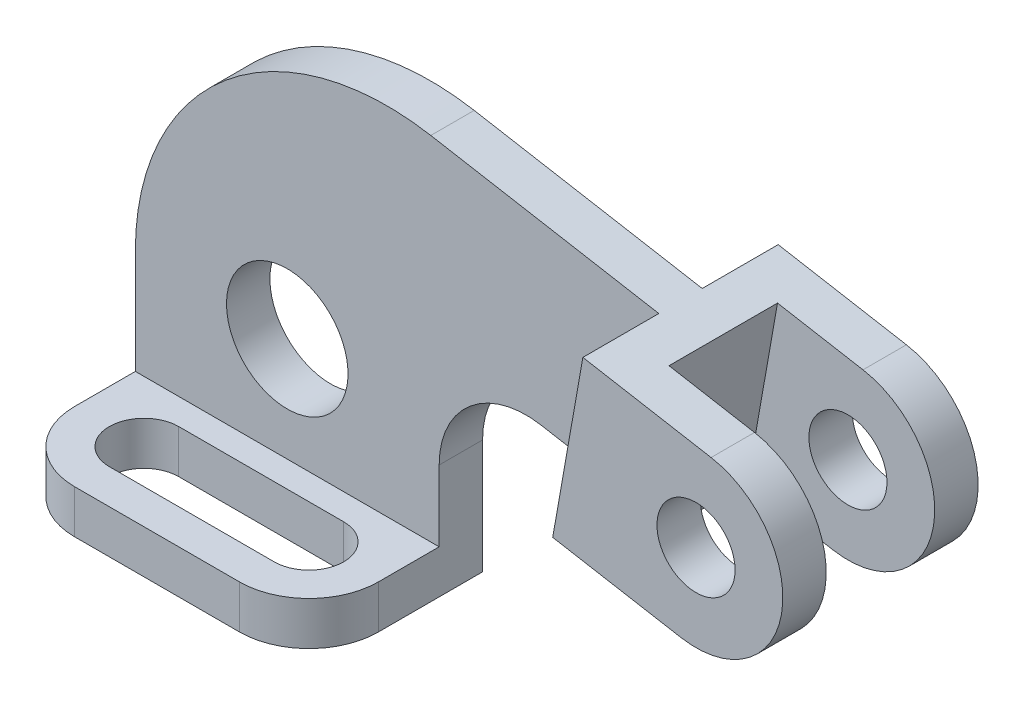
ISO-10303-21;
HEADER;
FILE_DESCRIPTION(('STEP AP214'),'2;1');
FILE_NAME('part.step','',(''),(''),'','','');
FILE_SCHEMA(('AUTOMOTIVE_DESIGN { 1 0 10303 214 1 1 1 1 }'));
ENDSEC;
DATA;
#1=APPLICATION_CONTEXT('core data for automotive mechanical design processes');
#2=APPLICATION_PROTOCOL_DEFINITION('international standard','automotive_design',2000,#1);
#3=PRODUCT_CONTEXT('',#1,'mechanical');
#4=PRODUCT('Part','Part','',(#3));
#5=PRODUCT_RELATED_PRODUCT_CATEGORY('part','',(#4));
#6=PRODUCT_DEFINITION_FORMATION('','',#4);
#7=PRODUCT_DEFINITION_CONTEXT('part definition',#1,'design');
#8=PRODUCT_DEFINITION('design','',#6,#7);
#9=PRODUCT_DEFINITION_SHAPE('','',#8);
#10=(LENGTH_UNIT() NAMED_UNIT(*) SI_UNIT(.MILLI.,.METRE.));
#11=(NAMED_UNIT(*) PLANE_ANGLE_UNIT() SI_UNIT($,.RADIAN.));
#12=(NAMED_UNIT(*) SI_UNIT($,.STERADIAN.) SOLID_ANGLE_UNIT());
#13=UNCERTAINTY_MEASURE_WITH_UNIT(LENGTH_MEASURE(1.E-05),#10,'distance_accuracy_value','');
#14=(GEOMETRIC_REPRESENTATION_CONTEXT(3) GLOBAL_UNCERTAINTY_ASSIGNED_CONTEXT((#13)) GLOBAL_UNIT_ASSIGNED_CONTEXT((#10,
#11,#12)) REPRESENTATION_CONTEXT('',''));
#15=CARTESIAN_POINT('',(0.,0.,0.));
#16=DIRECTION('',(0.,0.,1.));
#17=DIRECTION('',(1.,0.,0.));
#18=AXIS2_PLACEMENT_3D('',#15,#16,#17);
#19=CARTESIAN_POINT('',(-54.,10.,14.));
#20=DIRECTION('',(0.,1.,0.));
#21=DIRECTION('',(0.,0.,1.));
#22=AXIS2_PLACEMENT_3D('',#19,#20,#21);
#23=PLANE('',#22);
#24=DIRECTION('',(0.,0.,-1.));
#25=VECTOR('',#24,1.);
#26=CARTESIAN_POINT('',(0.,10.,13.9999999999999));
#27=LINE('',#26,#25);
#28=CARTESIAN_POINT('',(0.,10.,13.9999999999999));
#29=VERTEX_POINT('',#28);
#30=CARTESIAN_POINT('',(0.,10.,0.));
#31=VERTEX_POINT('',#30);
#32=EDGE_CURVE('E341',#29,#31,#27,.T.);
#33=ORIENTED_EDGE('',*,*,#32,.T.);
#34=DIRECTION('',(-1.,0.,0.));
#35=VECTOR('',#34,1.);
#36=CARTESIAN_POINT('',(0.,10.,0.));
#37=LINE('',#36,#35);
#38=CARTESIAN_POINT('',(-70.,10.,0.));
#39=VERTEX_POINT('',#38);
#40=EDGE_CURVE('E350',#31,#39,#37,.T.);
#41=ORIENTED_EDGE('',*,*,#40,.T.);
#42=DIRECTION('',(0.,0.,1.));
#43=VECTOR('',#42,1.);
#44=CARTESIAN_POINT('',(-70.,10.,0.));
#45=LINE('',#44,#43);
#46=CARTESIAN_POINT('',(-70.,10.,14.));
#47=VERTEX_POINT('',#46);
#48=EDGE_CURVE('E351',#39,#47,#45,.T.);
#49=ORIENTED_EDGE('',*,*,#48,.T.);
#50=CARTESIAN_POINT('',(-54.,10.,14.));
#51=DIRECTION('',(0.,1.,0.));
#52=DIRECTION('',(0.,0.,1.));
#53=AXIS2_PLACEMENT_3D('',#50,#51,#52);
#54=CIRCLE('',#53,16.);
#55=CARTESIAN_POINT('',(-54.,10.,30.));
#56=VERTEX_POINT('',#55);
#57=EDGE_CURVE('E354',#47,#56,#54,.T.);
#58=ORIENTED_EDGE('',*,*,#57,.T.);
#59=DIRECTION('',(1.,0.,0.));
#60=VECTOR('',#59,1.);
#61=CARTESIAN_POINT('',(-54.,10.,30.));
#62=LINE('',#61,#60);
#63=CARTESIAN_POINT('',(-16.0000000000001,10.,30.));
#64=VERTEX_POINT('',#63);
#65=EDGE_CURVE('E355',#56,#64,#62,.T.);
#66=ORIENTED_EDGE('',*,*,#65,.T.);
#67=CARTESIAN_POINT('',(-16.,10.,14.));
#68=DIRECTION('',(0.,1.,0.));
#69=DIRECTION('',(0.,0.,1.));
#70=AXIS2_PLACEMENT_3D('',#67,#68,#69);
#71=CIRCLE('',#70,16.);
#72=EDGE_CURVE('E360',#64,#29,#71,.T.);
#73=ORIENTED_EDGE('',*,*,#72,.T.);
#74=EDGE_LOOP('',(#33,#41,#49,#58,#66,#73));
#75=FACE_BOUND('',#74,.T.);
#76=DIRECTION('',(1.,0.,0.));
#77=VECTOR('',#76,1.);
#78=CARTESIAN_POINT('',(-54.,10.,22.));
#79=LINE('',#78,#77);
#80=CARTESIAN_POINT('',(-54.,10.,22.));
#81=VERTEX_POINT('',#80);
#82=CARTESIAN_POINT('',(-16.,10.,22.));
#83=VERTEX_POINT('',#82);
#84=EDGE_CURVE('E319',#81,#83,#79,.T.);
#85=ORIENTED_EDGE('',*,*,#84,.F.);
#86=CARTESIAN_POINT('',(-54.,10.,14.));
#87=DIRECTION('',(0.,1.,0.));
#88=DIRECTION('',(0.,0.,1.));
#89=AXIS2_PLACEMENT_3D('',#86,#87,#88);
#90=CIRCLE('',#89,8.);
#91=CARTESIAN_POINT('',(-54.,10.,6.00000000000001));
#92=VERTEX_POINT('',#91);
#93=EDGE_CURVE('E318',#92,#81,#90,.T.);
#94=ORIENTED_EDGE('',*,*,#93,.F.);
#95=DIRECTION('',(-1.,0.,0.));
#96=VECTOR('',#95,1.);
#97=CARTESIAN_POINT('',(-54.,10.,6.00000000000001));
#98=LINE('',#97,#96);
#99=CARTESIAN_POINT('',(-16.,10.,6.00000000000001));
#100=VERTEX_POINT('',#99);
#101=EDGE_CURVE('E324',#100,#92,#98,.T.);
#102=ORIENTED_EDGE('',*,*,#101,.F.);
#103=CARTESIAN_POINT('',(-16.,10.,14.));
#104=DIRECTION('',(0.,1.,0.));
#105=DIRECTION('',(0.,0.,1.));
#106=AXIS2_PLACEMENT_3D('',#103,#104,#105);
#107=CIRCLE('',#106,8.);
#108=EDGE_CURVE('E323',#83,#100,#107,.T.);
#109=ORIENTED_EDGE('',*,*,#108,.F.);
#110=EDGE_LOOP('',(#85,#94,#102,#109));
#111=FACE_BOUND('',#110,.T.);
#112=ADVANCED_FACE('F39',(#75,#111),#23,.T.);
#113=CARTESIAN_POINT('',(-54.,0.,14.));
#114=DIRECTION('',(0.,1.,0.));
#115=DIRECTION('',(0.,0.,1.));
#116=AXIS2_PLACEMENT_3D('',#113,#114,#115);
#117=PLANE('',#116);
#118=DIRECTION('',(0.,0.,-1.));
#119=VECTOR('',#118,1.);
#120=CARTESIAN_POINT('',(0.,0.,13.9999999999999));
#121=LINE('',#120,#119);
#122=CARTESIAN_POINT('',(0.,0.,13.9999999999999));
#123=VERTEX_POINT('',#122);
#124=CARTESIAN_POINT('',(0.,0.,-10.));
#125=VERTEX_POINT('',#124);
#126=EDGE_CURVE('E344',#123,#125,#121,.T.);
#127=ORIENTED_EDGE('',*,*,#126,.F.);
#128=CARTESIAN_POINT('',(-16.,0.,14.));
#129=DIRECTION('',(0.,1.,0.));
#130=DIRECTION('',(0.,0.,1.));
#131=AXIS2_PLACEMENT_3D('',#128,#129,#130);
#132=CIRCLE('',#131,16.);
#133=CARTESIAN_POINT('',(-16.0000000000001,0.,30.));
#134=VERTEX_POINT('',#133);
#135=EDGE_CURVE('E346',#134,#123,#132,.T.);
#136=ORIENTED_EDGE('',*,*,#135,.F.);
#137=DIRECTION('',(1.,0.,0.));
#138=VECTOR('',#137,1.);
#139=CARTESIAN_POINT('',(-54.,0.,30.));
#140=LINE('',#139,#138);
#141=CARTESIAN_POINT('',(-54.,0.,30.));
#142=VERTEX_POINT('',#141);
#143=EDGE_CURVE('E364',#142,#134,#140,.T.);
#144=ORIENTED_EDGE('',*,*,#143,.F.);
#145=CARTESIAN_POINT('',(-54.,0.,14.));
#146=DIRECTION('',(0.,1.,0.));
#147=DIRECTION('',(0.,0.,1.));
#148=AXIS2_PLACEMENT_3D('',#145,#146,#147);
#149=CIRCLE('',#148,16.);
#150=CARTESIAN_POINT('',(-70.,0.,14.));
#151=VERTEX_POINT('',#150);
#152=EDGE_CURVE('E361',#151,#142,#149,.T.);
#153=ORIENTED_EDGE('',*,*,#152,.F.);
#154=DIRECTION('',(0.,0.,1.));
#155=VECTOR('',#154,1.);
#156=CARTESIAN_POINT('',(-70.,0.,0.));
#157=LINE('',#156,#155);
#158=CARTESIAN_POINT('',(-70.,0.,-9.99999999999999));
#159=VERTEX_POINT('',#158);
#160=EDGE_CURVE('E363',#159,#151,#157,.T.);
#161=ORIENTED_EDGE('',*,*,#160,.F.);
#162=DIRECTION('',(-1.,0.,0.));
#163=VECTOR('',#162,1.);
#164=CARTESIAN_POINT('',(-70.,0.,-9.99999999999999));
#165=LINE('',#164,#163);
#166=EDGE_CURVE('E271',#125,#159,#165,.T.);
#167=ORIENTED_EDGE('',*,*,#166,.F.);
#168=EDGE_LOOP('',(#127,#136,#144,#153,#161,#167));
#169=FACE_BOUND('',#168,.T.);
#170=CARTESIAN_POINT('',(-54.,0.,14.));
#171=DIRECTION('',(0.,1.,0.));
#172=DIRECTION('',(0.,0.,1.));
#173=AXIS2_PLACEMENT_3D('',#170,#171,#172);
#174=CIRCLE('',#173,8.);
#175=CARTESIAN_POINT('',(-54.,0.,6.00000000000001));
#176=VERTEX_POINT('',#175);
#177=CARTESIAN_POINT('',(-54.,0.,22.));
#178=VERTEX_POINT('',#177);
#179=EDGE_CURVE('E62',#176,#178,#174,.T.);
#180=ORIENTED_EDGE('',*,*,#179,.T.);
#181=DIRECTION('',(1.,0.,0.));
#182=VECTOR('',#181,1.);
#183=CARTESIAN_POINT('',(-54.,0.,22.));
#184=LINE('',#183,#182);
#185=CARTESIAN_POINT('',(-16.,0.,22.));
#186=VERTEX_POINT('',#185);
#187=EDGE_CURVE('E328',#178,#186,#184,.T.);
#188=ORIENTED_EDGE('',*,*,#187,.T.);
#189=CARTESIAN_POINT('',(-16.,0.,14.));
#190=DIRECTION('',(0.,1.,0.));
#191=DIRECTION('',(0.,0.,1.));
#192=AXIS2_PLACEMENT_3D('',#189,#190,#191);
#193=CIRCLE('',#192,8.);
#194=CARTESIAN_POINT('',(-16.,0.,6.00000000000001));
#195=VERTEX_POINT('',#194);
#196=EDGE_CURVE('E335',#186,#195,#193,.T.);
#197=ORIENTED_EDGE('',*,*,#196,.T.);
#198=DIRECTION('',(-1.,0.,0.));
#199=VECTOR('',#198,1.);
#200=CARTESIAN_POINT('',(-54.,0.,6.00000000000001));
#201=LINE('',#200,#199);
#202=EDGE_CURVE('E321',#195,#176,#201,.T.);
#203=ORIENTED_EDGE('',*,*,#202,.T.);
#204=EDGE_LOOP('',(#180,#188,#197,#203));
#205=FACE_BOUND('',#204,.T.);
#206=ADVANCED_FACE('F384',(#169,#205),#117,.F.);
#207=CARTESIAN_POINT('',(0.,10.,13.9999999999999));
#208=DIRECTION('',(-1.,0.,0.));
#209=DIRECTION('',(0.,0.,1.));
#210=AXIS2_PLACEMENT_3D('',#207,#208,#209);
#211=PLANE('',#210);
#212=ORIENTED_EDGE('',*,*,#126,.T.);
#213=DIRECTION('',(0.,-1.,0.));
#214=VECTOR('',#213,1.);
#215=CARTESIAN_POINT('',(0.,0.,-10.));
#216=LINE('',#215,#214);
#217=CARTESIAN_POINT('',(0.,26.3266833935575,-10.));
#218=VERTEX_POINT('',#217);
#219=EDGE_CURVE('E286',#218,#125,#216,.T.);
#220=ORIENTED_EDGE('',*,*,#219,.F.);
#221=DIRECTION('',(0.,0.,1.));
#222=VECTOR('',#221,1.);
#223=CARTESIAN_POINT('',(0.,26.3266833935575,-10.));
#224=LINE('',#223,#222);
#225=CARTESIAN_POINT('',(0.,26.3266833935575,0.));
#226=VERTEX_POINT('',#225);
#227=EDGE_CURVE('E295',#218,#226,#224,.T.);
#228=ORIENTED_EDGE('',*,*,#227,.T.);
#229=DIRECTION('',(0.,-1.,0.));
#230=VECTOR('',#229,1.);
#231=CARTESIAN_POINT('',(0.,0.,0.));
#232=LINE('',#231,#230);
#233=EDGE_CURVE('E274',#226,#31,#232,.T.);
#234=ORIENTED_EDGE('',*,*,#233,.T.);
#235=ORIENTED_EDGE('',*,*,#32,.F.);
#236=DIRECTION('',(0.,-1.,0.));
#237=VECTOR('',#236,1.);
#238=CARTESIAN_POINT('',(0.,10.,13.9999999999999));
#239=LINE('',#238,#237);
#240=EDGE_CURVE('E356',#29,#123,#239,.T.);
#241=ORIENTED_EDGE('',*,*,#240,.T.);
#242=EDGE_LOOP('',(#212,#220,#228,#234,#235,#241));
#243=FACE_BOUND('',#242,.T.);
#244=ADVANCED_FACE('F41',(#243),#211,.F.);
#245=CARTESIAN_POINT('',(-70.,10.,0.));
#246=DIRECTION('',(1.,0.,0.));
#247=DIRECTION('',(0.,0.,-1.));
#248=AXIS2_PLACEMENT_3D('',#245,#246,#247);
#249=PLANE('',#248);
#250=ORIENTED_EDGE('',*,*,#160,.T.);
#251=DIRECTION('',(0.,-1.,0.));
#252=VECTOR('',#251,1.);
#253=CARTESIAN_POINT('',(-70.,10.,14.));
#254=LINE('',#253,#252);
#255=EDGE_CURVE('E11',#47,#151,#254,.T.);
#256=ORIENTED_EDGE('',*,*,#255,.F.);
#257=ORIENTED_EDGE('',*,*,#48,.F.);
#258=DIRECTION('',(0.,1.,0.));
#259=VECTOR('',#258,1.);
#260=CARTESIAN_POINT('',(-70.,0.,0.));
#261=LINE('',#260,#259);
#262=CARTESIAN_POINT('',(-70.,34.,0.));
#263=VERTEX_POINT('',#262);
#264=EDGE_CURVE('E268',#39,#263,#261,.T.);
#265=ORIENTED_EDGE('',*,*,#264,.T.);
#266=DIRECTION('',(0.,0.,1.));
#267=VECTOR('',#266,1.);
#268=CARTESIAN_POINT('',(-70.,34.,-9.99999999999999));
#269=LINE('',#268,#267);
#270=CARTESIAN_POINT('',(-70.,34.,-9.99999999999999));
#271=VERTEX_POINT('',#270);
#272=EDGE_CURVE('E312',#271,#263,#269,.T.);
#273=ORIENTED_EDGE('',*,*,#272,.F.);
#274=DIRECTION('',(0.,1.,0.));
#275=VECTOR('',#274,1.);
#276=CARTESIAN_POINT('',(-70.,0.,-9.99999999999999));
#277=LINE('',#276,#275);
#278=EDGE_CURVE('E273',#159,#271,#277,.T.);
#279=ORIENTED_EDGE('',*,*,#278,.F.);
#280=EDGE_LOOP('',(#250,#256,#257,#265,#273,#279));
#281=FACE_BOUND('',#280,.T.);
#282=ADVANCED_FACE('F405',(#281),#249,.F.);
#283=CARTESIAN_POINT('',(-54.,10.,14.));
#284=DIRECTION('',(0.,-1.,0.));
#285=DIRECTION('',(0.,0.,-1.));
#286=AXIS2_PLACEMENT_3D('',#283,#284,#285);
#287=CYLINDRICAL_SURFACE('',#286,16.);
#288=ORIENTED_EDGE('',*,*,#152,.T.);
#289=DIRECTION('',(0.,-1.,0.));
#290=VECTOR('',#289,1.);
#291=CARTESIAN_POINT('',(-54.,10.,30.));
#292=LINE('',#291,#290);
#293=EDGE_CURVE('E50',#56,#142,#292,.T.);
#294=ORIENTED_EDGE('',*,*,#293,.F.);
#295=ORIENTED_EDGE('',*,*,#57,.F.);
#296=ORIENTED_EDGE('',*,*,#255,.T.);
#297=EDGE_LOOP('',(#288,#294,#295,#296));
#298=FACE_BOUND('',#297,.T.);
#299=ADVANCED_FACE('F398',(#298),#287,.T.);
#300=CARTESIAN_POINT('',(-54.,10.,30.));
#301=DIRECTION('',(0.,0.,-1.));
#302=DIRECTION('',(-1.,0.,0.));
#303=AXIS2_PLACEMENT_3D('',#300,#301,#302);
#304=PLANE('',#303);
#305=ORIENTED_EDGE('',*,*,#143,.T.);
#306=DIRECTION('',(0.,-1.,0.));
#307=VECTOR('',#306,1.);
#308=CARTESIAN_POINT('',(-16.0000000000001,10.,30.));
#309=LINE('',#308,#307);
#310=EDGE_CURVE('E367',#64,#134,#309,.T.);
#311=ORIENTED_EDGE('',*,*,#310,.F.);
#312=ORIENTED_EDGE('',*,*,#65,.F.);
#313=ORIENTED_EDGE('',*,*,#293,.T.);
#314=EDGE_LOOP('',(#305,#311,#312,#313));
#315=FACE_BOUND('',#314,.T.);
#316=ADVANCED_FACE('F380',(#315),#304,.F.);
#317=CARTESIAN_POINT('',(-16.,10.,14.));
#318=DIRECTION('',(0.,-1.,0.));
#319=DIRECTION('',(0.,0.,-1.));
#320=AXIS2_PLACEMENT_3D('',#317,#318,#319);
#321=CYLINDRICAL_SURFACE('',#320,16.);
#322=ORIENTED_EDGE('',*,*,#135,.T.);
#323=ORIENTED_EDGE('',*,*,#240,.F.);
#324=ORIENTED_EDGE('',*,*,#72,.F.);
#325=ORIENTED_EDGE('',*,*,#310,.T.);
#326=EDGE_LOOP('',(#322,#323,#324,#325));
#327=FACE_BOUND('',#326,.T.);
#328=ADVANCED_FACE('F388',(#327),#321,.T.);
#329=CARTESIAN_POINT('',(-54.,10.,14.));
#330=DIRECTION('',(0.,-1.,0.));
#331=DIRECTION('',(0.,0.,-1.));
#332=AXIS2_PLACEMENT_3D('',#329,#330,#331);
#333=CYLINDRICAL_SURFACE('',#332,8.);
#334=ORIENTED_EDGE('',*,*,#179,.F.);
#335=DIRECTION('',(0.,-1.,0.));
#336=VECTOR('',#335,1.);
#337=CARTESIAN_POINT('',(-54.,10.,6.00000000000001));
#338=LINE('',#337,#336);
#339=EDGE_CURVE('E330',#92,#176,#338,.T.);
#340=ORIENTED_EDGE('',*,*,#339,.F.);
#341=ORIENTED_EDGE('',*,*,#93,.T.);
#342=DIRECTION('',(0.,-1.,0.));
#343=VECTOR('',#342,1.);
#344=CARTESIAN_POINT('',(-54.,10.,22.));
#345=LINE('',#344,#343);
#346=EDGE_CURVE('E342',#81,#178,#345,.T.);
#347=ORIENTED_EDGE('',*,*,#346,.T.);
#348=EDGE_LOOP('',(#334,#340,#341,#347));
#349=FACE_BOUND('',#348,.T.);
#350=ADVANCED_FACE('F495',(#349),#333,.F.);
#351=CARTESIAN_POINT('',(-54.,10.,22.));
#352=DIRECTION('',(0.,0.,-1.));
#353=DIRECTION('',(-1.,0.,0.));
#354=AXIS2_PLACEMENT_3D('',#351,#352,#353);
#355=PLANE('',#354);
#356=ORIENTED_EDGE('',*,*,#187,.F.);
#357=ORIENTED_EDGE('',*,*,#346,.F.);
#358=ORIENTED_EDGE('',*,*,#84,.T.);
#359=DIRECTION('',(0.,-1.,0.));
#360=VECTOR('',#359,1.);
#361=CARTESIAN_POINT('',(-16.,10.,22.));
#362=LINE('',#361,#360);
#363=EDGE_CURVE('E338',#83,#186,#362,.T.);
#364=ORIENTED_EDGE('',*,*,#363,.T.);
#365=EDGE_LOOP('',(#356,#357,#358,#364));
#366=FACE_BOUND('',#365,.T.);
#367=ADVANCED_FACE('F534',(#366),#355,.T.);
#368=CARTESIAN_POINT('',(-16.,10.,14.));
#369=DIRECTION('',(0.,-1.,0.));
#370=DIRECTION('',(0.,0.,-1.));
#371=AXIS2_PLACEMENT_3D('',#368,#369,#370);
#372=CYLINDRICAL_SURFACE('',#371,8.);
#373=ORIENTED_EDGE('',*,*,#196,.F.);
#374=ORIENTED_EDGE('',*,*,#363,.F.);
#375=ORIENTED_EDGE('',*,*,#108,.T.);
#376=DIRECTION('',(0.,-1.,0.));
#377=VECTOR('',#376,1.);
#378=CARTESIAN_POINT('',(-16.,10.,6.00000000000001));
#379=LINE('',#378,#377);
#380=EDGE_CURVE('E53',#100,#195,#379,.T.);
#381=ORIENTED_EDGE('',*,*,#380,.T.);
#382=EDGE_LOOP('',(#373,#374,#375,#381));
#383=FACE_BOUND('',#382,.T.);
#384=ADVANCED_FACE('F521',(#383),#372,.F.);
#385=CARTESIAN_POINT('',(-54.,10.,6.00000000000001));
#386=DIRECTION('',(0.,0.,1.));
#387=DIRECTION('',(1.,0.,0.));
#388=AXIS2_PLACEMENT_3D('',#385,#386,#387);
#389=PLANE('',#388);
#390=ORIENTED_EDGE('',*,*,#202,.F.);
#391=ORIENTED_EDGE('',*,*,#380,.F.);
#392=ORIENTED_EDGE('',*,*,#101,.T.);
#393=ORIENTED_EDGE('',*,*,#339,.T.);
#394=EDGE_LOOP('',(#390,#391,#392,#393));
#395=FACE_BOUND('',#394,.T.);
#396=ADVANCED_FACE('F518',(#395),#389,.T.);
#397=CARTESIAN_POINT('',(20.,26.3266833935575,-10.));
#398=DIRECTION('',(0.,0.,-1.));
#399=DIRECTION('',(-1.,0.,0.));
#400=AXIS2_PLACEMENT_3D('',#397,#398,#399);
#401=PLANE('',#400);
#402=ORIENTED_EDGE('',*,*,#166,.T.);
#403=ORIENTED_EDGE('',*,*,#278,.T.);
#404=CARTESIAN_POINT('',(-12.,34.,-10.));
#405=DIRECTION('',(0.,0.,-1.));
#406=DIRECTION('',(-1.,0.,0.));
#407=AXIS2_PLACEMENT_3D('',#404,#405,#406);
#408=CIRCLE('',#407,58.);
#409=CARTESIAN_POINT('',(-1.92840569531779,91.118849674708,-10.));
#410=VERTEX_POINT('',#409);
#411=EDGE_CURVE('E280',#271,#410,#408,.T.);
#412=ORIENTED_EDGE('',*,*,#411,.T.);
#413=DIRECTION('',(0.984807753012207,-0.173648177666935,0.));
#414=VECTOR('',#413,1.);
#415=CARTESIAN_POINT('',(-1.92840569531779,91.118849674708,-10.));
#416=LINE('',#415,#414);
#417=CARTESIAN_POINT('',(50.610518394572,81.8548198202663,-10.));
#418=VERTEX_POINT('',#417);
#419=EDGE_CURVE('E276',#410,#418,#416,.T.);
#420=ORIENTED_EDGE('',*,*,#419,.T.);
#421=DIRECTION('',(-0.173648177666935,-0.984807753012207,0.));
#422=VECTOR('',#421,1.);
#423=CARTESIAN_POINT('',(50.610518394572,81.8548198202663,-10.));
#424=LINE('',#423,#422);
#425=CARTESIAN_POINT('',(43.6645912878946,42.462509699778,-10.));
#426=VERTEX_POINT('',#425);
#427=EDGE_CURVE('E282',#418,#426,#424,.T.);
#428=ORIENTED_EDGE('',*,*,#427,.T.);
#429=DIRECTION('',(-0.984807753012207,0.173648177666934,0.));
#430=VECTOR('',#429,1.);
#431=CARTESIAN_POINT('',(23.4729635533387,46.0228384538016,-10.));
#432=LINE('',#431,#430);
#433=CARTESIAN_POINT('',(23.4729635533387,46.0228384538016,-10.));
#434=VERTEX_POINT('',#433);
#435=EDGE_CURVE('E285',#426,#434,#432,.T.);
#436=ORIENTED_EDGE('',*,*,#435,.T.);
#437=CARTESIAN_POINT('',(20.,26.3266833935575,-10.));
#438=DIRECTION('',(0.,0.,1.));
#439=DIRECTION('',(-1.,0.,0.));
#440=AXIS2_PLACEMENT_3D('',#437,#438,#439);
#441=CIRCLE('',#440,20.);
#442=EDGE_CURVE('E290',#434,#218,#441,.T.);
#443=ORIENTED_EDGE('',*,*,#442,.T.);
#444=ORIENTED_EDGE('',*,*,#219,.T.);
#445=EDGE_LOOP('',(#402,#403,#412,#420,#428,#436,#443,#444));
#446=FACE_BOUND('',#445,.T.);
#447=CARTESIAN_POINT('',(-35.,34.,-10.));
#448=DIRECTION('',(0.,0.,-1.));
#449=DIRECTION('',(-1.,0.,0.));
#450=AXIS2_PLACEMENT_3D('',#447,#448,#449);
#451=CIRCLE('',#450,14.);
#452=CARTESIAN_POINT('',(-49.,34.,-9.99999999999999));
#453=VERTEX_POINT('',#452);
#454=EDGE_CURVE('E264',#453,#453,#451,.T.);
#455=ORIENTED_EDGE('',*,*,#454,.F.);
#456=EDGE_LOOP('',(#455));
#457=FACE_BOUND('',#456,.T.);
#458=ADVANCED_FACE('F406',(#446,#457),#401,.T.);
#459=CARTESIAN_POINT('',(20.,26.3266833935575,0.));
#460=DIRECTION('',(0.,0.,-1.));
#461=DIRECTION('',(-1.,0.,0.));
#462=AXIS2_PLACEMENT_3D('',#459,#460,#461);
#463=PLANE('',#462);
#464=ORIENTED_EDGE('',*,*,#40,.F.);
#465=ORIENTED_EDGE('',*,*,#233,.F.);
#466=CARTESIAN_POINT('',(20.,26.3266833935575,0.));
#467=DIRECTION('',(0.,0.,1.));
#468=DIRECTION('',(-1.,0.,0.));
#469=AXIS2_PLACEMENT_3D('',#466,#467,#468);
#470=CIRCLE('',#469,20.);
#471=CARTESIAN_POINT('',(23.4729635533387,46.0228384538016,0.));
#472=VERTEX_POINT('',#471);
#473=EDGE_CURVE('E304',#472,#226,#470,.T.);
#474=ORIENTED_EDGE('',*,*,#473,.F.);
#475=DIRECTION('',(-0.984807753012207,0.173648177666934,0.));
#476=VECTOR('',#475,1.);
#477=CARTESIAN_POINT('',(23.4729635533387,46.0228384538016,0.));
#478=LINE('',#477,#476);
#479=CARTESIAN_POINT('',(43.6645912878946,42.462509699778,0.));
#480=VERTEX_POINT('',#479);
#481=EDGE_CURVE('E302',#480,#472,#478,.T.);
#482=ORIENTED_EDGE('',*,*,#481,.F.);
#483=DIRECTION('',(-0.173648177666935,-0.984807753012207,0.));
#484=VECTOR('',#483,1.);
#485=CARTESIAN_POINT('',(50.610518394572,81.8548198202663,0.));
#486=LINE('',#485,#484);
#487=CARTESIAN_POINT('',(50.610518394572,81.8548198202663,0.));
#488=VERTEX_POINT('',#487);
#489=EDGE_CURVE('E298',#488,#480,#486,.T.);
#490=ORIENTED_EDGE('',*,*,#489,.F.);
#491=DIRECTION('',(0.984807753012207,-0.173648177666935,0.));
#492=VECTOR('',#491,1.);
#493=CARTESIAN_POINT('',(-1.92840569531779,91.118849674708,0.));
#494=LINE('',#493,#492);
#495=CARTESIAN_POINT('',(-1.92840569531779,91.118849674708,0.));
#496=VERTEX_POINT('',#495);
#497=EDGE_CURVE('E296',#496,#488,#494,.T.);
#498=ORIENTED_EDGE('',*,*,#497,.F.);
#499=CARTESIAN_POINT('',(-12.,34.,0.));
#500=DIRECTION('',(0.,0.,-1.));
#501=DIRECTION('',(-1.,0.,0.));
#502=AXIS2_PLACEMENT_3D('',#499,#500,#501);
#503=CIRCLE('',#502,58.);
#504=EDGE_CURVE('E294',#263,#496,#503,.T.);
#505=ORIENTED_EDGE('',*,*,#504,.F.);
#506=ORIENTED_EDGE('',*,*,#264,.F.);
#507=EDGE_LOOP('',(#464,#465,#474,#482,#490,#498,#505,#506));
#508=FACE_BOUND('',#507,.T.);
#509=CARTESIAN_POINT('',(-35.,34.,0.));
#510=DIRECTION('',(0.,0.,-1.));
#511=DIRECTION('',(-1.,0.,0.));
#512=AXIS2_PLACEMENT_3D('',#509,#510,#511);
#513=CIRCLE('',#512,14.);
#514=CARTESIAN_POINT('',(-49.,34.,0.));
#515=VERTEX_POINT('',#514);
#516=EDGE_CURVE('E259',#515,#515,#513,.T.);
#517=ORIENTED_EDGE('',*,*,#516,.T.);
#518=EDGE_LOOP('',(#517));
#519=FACE_BOUND('',#518,.T.);
#520=ADVANCED_FACE('F414',(#508,#519),#463,.F.);
#521=CARTESIAN_POINT('',(-12.,34.,-10.));
#522=DIRECTION('',(0.,0.,1.));
#523=DIRECTION('',(1.,0.,0.));
#524=AXIS2_PLACEMENT_3D('',#521,#522,#523);
#525=CYLINDRICAL_SURFACE('',#524,58.);
#526=ORIENTED_EDGE('',*,*,#504,.T.);
#527=DIRECTION('',(0.,0.,1.));
#528=VECTOR('',#527,1.);
#529=CARTESIAN_POINT('',(-1.92840569531779,91.118849674708,-10.));
#530=LINE('',#529,#528);
#531=EDGE_CURVE('E315',#410,#496,#530,.T.);
#532=ORIENTED_EDGE('',*,*,#531,.F.);
#533=ORIENTED_EDGE('',*,*,#411,.F.);
#534=ORIENTED_EDGE('',*,*,#272,.T.);
#535=EDGE_LOOP('',(#526,#532,#533,#534));
#536=FACE_BOUND('',#535,.T.);
#537=ADVANCED_FACE('F419',(#536),#525,.T.);
#538=CARTESIAN_POINT('',(-1.92840569531779,91.118849674708,-10.));
#539=DIRECTION('',(-0.173648177666935,-0.984807753012207,0.));
#540=DIRECTION('',(0.984807753012207,-0.173648177666935,0.));
#541=AXIS2_PLACEMENT_3D('',#538,#539,#540);
#542=PLANE('',#541);
#543=ORIENTED_EDGE('',*,*,#497,.T.);
#544=DIRECTION('',(0.,0.,1.));
#545=VECTOR('',#544,1.);
#546=CARTESIAN_POINT('',(50.610518394572,81.8548198202663,-27.5));
#547=LINE('',#546,#545);
#548=CARTESIAN_POINT('',(50.6105183945721,81.8548198202663,17.5));
#549=VERTEX_POINT('',#548);
#550=EDGE_CURVE('E239',#488,#549,#547,.T.);
#551=ORIENTED_EDGE('',*,*,#550,.T.);
#552=DIRECTION('',(0.984807753012207,-0.173648177666935,0.));
#553=VECTOR('',#552,1.);
#554=CARTESIAN_POINT('',(50.6105183945721,81.8548198202663,17.5));
#555=LINE('',#554,#553);
#556=CARTESIAN_POINT('',(80.1547509849383,76.6453744902582,17.5));
#557=VERTEX_POINT('',#556);
#558=EDGE_CURVE('E236',#549,#557,#555,.T.);
#559=ORIENTED_EDGE('',*,*,#558,.T.);
#560=DIRECTION('',(0.,0.,-1.));
#561=VECTOR('',#560,1.);
#562=CARTESIAN_POINT('',(80.1547509849383,76.6453744902582,17.5));
#563=LINE('',#562,#561);
#564=CARTESIAN_POINT('',(80.1547509849382,76.6453744902582,7.5));
#565=VERTEX_POINT('',#564);
#566=EDGE_CURVE('E241',#557,#565,#563,.T.);
#567=ORIENTED_EDGE('',*,*,#566,.T.);
#568=DIRECTION('',(-0.984807753012207,0.173648177666935,0.));
#569=VECTOR('',#568,1.);
#570=CARTESIAN_POINT('',(60.4585959246941,80.1183380435969,7.5));
#571=LINE('',#570,#569);
#572=CARTESIAN_POINT('',(60.4585959246941,80.1183380435969,7.5));
#573=VERTEX_POINT('',#572);
#574=EDGE_CURVE('E243',#565,#573,#571,.T.);
#575=ORIENTED_EDGE('',*,*,#574,.T.);
#576=DIRECTION('',(0.,0.,-1.));
#577=VECTOR('',#576,1.);
#578=CARTESIAN_POINT('',(60.4585959246941,80.1183380435969,-17.5));
#579=LINE('',#578,#577);
#580=CARTESIAN_POINT('',(60.4585959246941,80.1183380435969,-17.5));
#581=VERTEX_POINT('',#580);
#582=EDGE_CURVE('E250',#573,#581,#579,.T.);
#583=ORIENTED_EDGE('',*,*,#582,.T.);
#584=DIRECTION('',(0.984807753012207,-0.173648177666935,0.));
#585=VECTOR('',#584,1.);
#586=CARTESIAN_POINT('',(60.4585959246941,80.1183380435969,-17.5));
#587=LINE('',#586,#585);
#588=CARTESIAN_POINT('',(80.1547509849382,76.6453744902582,-17.5));
#589=VERTEX_POINT('',#588);
#590=EDGE_CURVE('E248',#581,#589,#587,.T.);
#591=ORIENTED_EDGE('',*,*,#590,.T.);
#592=DIRECTION('',(0.,0.,-1.));
#593=VECTOR('',#592,1.);
#594=CARTESIAN_POINT('',(80.1547509849383,76.6453744902582,-27.5));
#595=LINE('',#594,#593);
#596=CARTESIAN_POINT('',(80.1547509849383,76.6453744902582,-27.5));
#597=VERTEX_POINT('',#596);
#598=EDGE_CURVE('E210',#589,#597,#595,.T.);
#599=ORIENTED_EDGE('',*,*,#598,.T.);
#600=DIRECTION('',(-0.984807753012207,0.173648177666935,0.));
#601=VECTOR('',#600,1.);
#602=CARTESIAN_POINT('',(50.610518394572,81.8548198202663,-27.5));
#603=LINE('',#602,#601);
#604=CARTESIAN_POINT('',(50.610518394572,81.8548198202663,-27.5));
#605=VERTEX_POINT('',#604);
#606=EDGE_CURVE('E251',#597,#605,#603,.T.);
#607=ORIENTED_EDGE('',*,*,#606,.T.);
#608=EDGE_CURVE('E233',#605,#418,#547,.T.);
#609=ORIENTED_EDGE('',*,*,#608,.T.);
#610=ORIENTED_EDGE('',*,*,#419,.F.);
#611=ORIENTED_EDGE('',*,*,#531,.T.);
#612=EDGE_LOOP('',(#543,#551,#559,#567,#575,#583,#591,#599,#607,#609,#610,#611));
#613=FACE_BOUND('',#612,.T.);
#614=ADVANCED_FACE('F422',(#613),#542,.F.);
#615=CARTESIAN_POINT('',(23.4729635533387,46.0228384538016,-10.));
#616=DIRECTION('',(0.173648177666934,0.984807753012207,0.));
#617=DIRECTION('',(-0.984807753012208,0.173648177666934,0.));
#618=AXIS2_PLACEMENT_3D('',#615,#616,#617);
#619=PLANE('',#618);
#620=ORIENTED_EDGE('',*,*,#481,.T.);
#621=DIRECTION('',(0.,0.,1.));
#622=VECTOR('',#621,1.);
#623=CARTESIAN_POINT('',(23.4729635533387,46.0228384538016,-10.));
#624=LINE('',#623,#622);
#625=EDGE_CURVE('E310',#434,#472,#624,.T.);
#626=ORIENTED_EDGE('',*,*,#625,.F.);
#627=ORIENTED_EDGE('',*,*,#435,.F.);
#628=DIRECTION('',(0.,0.,1.));
#629=VECTOR('',#628,1.);
#630=CARTESIAN_POINT('',(43.6645912878946,42.462509699778,-27.5));
#631=LINE('',#630,#629);
#632=CARTESIAN_POINT('',(43.6645912878946,42.462509699778,-27.5));
#633=VERTEX_POINT('',#632);
#634=EDGE_CURVE('E431',#633,#426,#631,.T.);
#635=ORIENTED_EDGE('',*,*,#634,.F.);
#636=DIRECTION('',(-0.984807753012207,0.173648177666934,0.));
#637=VECTOR('',#636,1.);
#638=CARTESIAN_POINT('',(53.5126688180167,40.7260279231086,-27.5));
#639=LINE('',#638,#637);
#640=CARTESIAN_POINT('',(73.2088238782608,37.25306436977,-27.5));
#641=VERTEX_POINT('',#640);
#642=EDGE_CURVE('E224',#641,#633,#639,.T.);
#643=ORIENTED_EDGE('',*,*,#642,.F.);
#644=DIRECTION('',(0.,0.,-1.));
#645=VECTOR('',#644,1.);
#646=CARTESIAN_POINT('',(73.2088238782609,37.2530643697699,-27.5));
#647=LINE('',#646,#645);
#648=CARTESIAN_POINT('',(73.2088238782609,37.25306436977,-17.5));
#649=VERTEX_POINT('',#648);
#650=EDGE_CURVE('E204',#649,#641,#647,.T.);
#651=ORIENTED_EDGE('',*,*,#650,.F.);
#652=DIRECTION('',(0.984807753012207,-0.173648177666935,0.));
#653=VECTOR('',#652,1.);
#654=CARTESIAN_POINT('',(53.5126688180167,40.7260279231086,-17.5));
#655=LINE('',#654,#653);
#656=CARTESIAN_POINT('',(53.5126688180167,40.7260279231086,-17.5));
#657=VERTEX_POINT('',#656);
#658=EDGE_CURVE('E219',#657,#649,#655,.T.);
#659=ORIENTED_EDGE('',*,*,#658,.F.);
#660=DIRECTION('',(0.,0.,-1.));
#661=VECTOR('',#660,1.);
#662=CARTESIAN_POINT('',(53.5126688180167,40.7260279231086,-17.5));
#663=LINE('',#662,#661);
#664=CARTESIAN_POINT('',(53.5126688180167,40.7260279231086,7.5));
#665=VERTEX_POINT('',#664);
#666=EDGE_CURVE('E227',#665,#657,#663,.T.);
#667=ORIENTED_EDGE('',*,*,#666,.F.);
#668=DIRECTION('',(-0.984807753012207,0.173648177666935,0.));
#669=VECTOR('',#668,1.);
#670=CARTESIAN_POINT('',(53.5126688180167,40.7260279231086,7.5));
#671=LINE('',#670,#669);
#672=CARTESIAN_POINT('',(73.2088238782608,37.25306436977,7.5));
#673=VERTEX_POINT('',#672);
#674=EDGE_CURVE('E228',#673,#665,#671,.T.);
#675=ORIENTED_EDGE('',*,*,#674,.F.);
#676=DIRECTION('',(0.,0.,-1.));
#677=VECTOR('',#676,1.);
#678=CARTESIAN_POINT('',(73.2088238782609,37.2530643697699,17.5));
#679=LINE('',#678,#677);
#680=CARTESIAN_POINT('',(73.2088238782609,37.2530643697699,17.5));
#681=VERTEX_POINT('',#680);
#682=EDGE_CURVE('E434',#681,#673,#679,.T.);
#683=ORIENTED_EDGE('',*,*,#682,.F.);
#684=DIRECTION('',(0.984807753012207,-0.173648177666935,0.));
#685=VECTOR('',#684,1.);
#686=CARTESIAN_POINT('',(43.6645912878947,42.462509699778,17.5));
#687=LINE('',#686,#685);
#688=CARTESIAN_POINT('',(43.6645912878947,42.462509699778,17.5));
#689=VERTEX_POINT('',#688);
#690=EDGE_CURVE('E435',#689,#681,#687,.T.);
#691=ORIENTED_EDGE('',*,*,#690,.F.);
#692=EDGE_CURVE('E258',#480,#689,#631,.T.);
#693=ORIENTED_EDGE('',*,*,#692,.F.);
#694=EDGE_LOOP('',(#620,#626,#627,#635,#643,#651,#659,#667,#675,#683,#691,#693));
#695=FACE_BOUND('',#694,.T.);
#696=ADVANCED_FACE('F217',(#695),#619,.F.);
#697=CARTESIAN_POINT('',(20.,26.3266833935575,-10.));
#698=DIRECTION('',(0.,0.,1.));
#699=DIRECTION('',(1.,0.,0.));
#700=AXIS2_PLACEMENT_3D('',#697,#698,#699);
#701=CYLINDRICAL_SURFACE('',#700,20.);
#702=ORIENTED_EDGE('',*,*,#473,.T.);
#703=ORIENTED_EDGE('',*,*,#227,.F.);
#704=ORIENTED_EDGE('',*,*,#442,.F.);
#705=ORIENTED_EDGE('',*,*,#625,.T.);
#706=EDGE_LOOP('',(#702,#703,#704,#705));
#707=FACE_BOUND('',#706,.T.);
#708=ADVANCED_FACE('F630',(#707),#701,.F.);
#709=CARTESIAN_POINT('',(-35.,34.,-10.));
#710=DIRECTION('',(0.,0.,1.));
#711=DIRECTION('',(1.,0.,0.));
#712=AXIS2_PLACEMENT_3D('',#709,#710,#711);
#713=CYLINDRICAL_SURFACE('',#712,14.);
#714=ORIENTED_EDGE('',*,*,#454,.T.);
#715=EDGE_LOOP('',(#714));
#716=FACE_BOUND('',#715,.T.);
#717=ORIENTED_EDGE('',*,*,#516,.F.);
#718=EDGE_LOOP('',(#717));
#719=FACE_BOUND('',#718,.T.);
#720=ADVANCED_FACE('F640',(#716,#719),#713,.F.);
#721=CARTESIAN_POINT('',(43.6645912878946,42.462509699778,-27.5));
#722=DIRECTION('',(-0.984807753012207,0.173648177666935,0.));
#723=DIRECTION('',(-0.173648177666935,-0.984807753012207,0.));
#724=AXIS2_PLACEMENT_3D('',#721,#722,#723);
#725=PLANE('',#724);
#726=ORIENTED_EDGE('',*,*,#427,.F.);
#727=ORIENTED_EDGE('',*,*,#608,.F.);
#728=DIRECTION('',(0.173648177666935,0.984807753012207,0.));
#729=VECTOR('',#728,1.);
#730=CARTESIAN_POINT('',(43.6645912878946,42.462509699778,-27.5));
#731=LINE('',#730,#729);
#732=EDGE_CURVE('E260',#633,#605,#731,.T.);
#733=ORIENTED_EDGE('',*,*,#732,.F.);
#734=ORIENTED_EDGE('',*,*,#634,.T.);
#735=EDGE_LOOP('',(#726,#727,#733,#734));
#736=FACE_BOUND('',#735,.T.);
#737=ADVANCED_FACE('F429',(#736),#725,.T.);
#738=ORIENTED_EDGE('',*,*,#550,.F.);
#739=ORIENTED_EDGE('',*,*,#489,.T.);
#740=ORIENTED_EDGE('',*,*,#692,.T.);
#741=DIRECTION('',(0.173648177666935,0.984807753012207,0.));
#742=VECTOR('',#741,1.);
#743=CARTESIAN_POINT('',(43.6645912878947,42.462509699778,17.5));
#744=LINE('',#743,#742);
#745=EDGE_CURVE('E231',#689,#549,#744,.T.);
#746=ORIENTED_EDGE('',*,*,#745,.T.);
#747=EDGE_LOOP('',(#738,#739,#740,#746));
#748=FACE_BOUND('',#747,.T.);
#749=ADVANCED_FACE('F653',(#748),#725,.T.);
#750=CARTESIAN_POINT('',(43.6645912878946,42.462509699778,-27.5));
#751=DIRECTION('',(0.,0.,-1.));
#752=DIRECTION('',(0.,1.,0.));
#753=AXIS2_PLACEMENT_3D('',#750,#751,#752);
#754=PLANE('',#753);
#755=CARTESIAN_POINT('',(76.6817874315996,56.9492194300141,-27.5));
#756=DIRECTION('',(0.,0.,1.));
#757=DIRECTION('',(1.,0.,0.));
#758=AXIS2_PLACEMENT_3D('',#755,#756,#757);
#759=CIRCLE('',#758,9.);
#760=CARTESIAN_POINT('',(85.6817874315996,56.9492194300141,-27.5));
#761=VERTEX_POINT('',#760);
#762=EDGE_CURVE('E463',#761,#761,#759,.T.);
#763=ORIENTED_EDGE('',*,*,#762,.T.);
#764=EDGE_LOOP('',(#763));
#765=FACE_BOUND('',#764,.T.);
#766=ORIENTED_EDGE('',*,*,#606,.F.);
#767=CARTESIAN_POINT('',(76.6817874315996,56.9492194300141,-27.5));
#768=DIRECTION('',(0.,0.,-1.));
#769=DIRECTION('',(0.,1.,0.));
#770=AXIS2_PLACEMENT_3D('',#767,#768,#769);
#771=CIRCLE('',#770,20.);
#772=EDGE_CURVE('E213',#597,#641,#771,.T.);
#773=ORIENTED_EDGE('',*,*,#772,.T.);
#774=ORIENTED_EDGE('',*,*,#642,.T.);
#775=ORIENTED_EDGE('',*,*,#732,.T.);
#776=EDGE_LOOP('',(#766,#773,#774,#775));
#777=FACE_BOUND('',#776,.T.);
#778=ADVANCED_FACE('F473',(#765,#777),#754,.T.);
#779=CARTESIAN_POINT('',(53.5126688180167,40.7260279231086,-17.5));
#780=DIRECTION('',(0.,0.,1.));
#781=DIRECTION('',(0.,-1.,0.));
#782=AXIS2_PLACEMENT_3D('',#779,#780,#781);
#783=PLANE('',#782);
#784=CARTESIAN_POINT('',(76.6817874315996,56.9492194300141,-17.5));
#785=DIRECTION('',(0.,0.,1.));
#786=DIRECTION('',(0.,-1.,0.));
#787=AXIS2_PLACEMENT_3D('',#784,#785,#786);
#788=CIRCLE('',#787,9.);
#789=CARTESIAN_POINT('',(85.6817874315996,56.9492194300141,-17.5));
#790=VERTEX_POINT('',#789);
#791=EDGE_CURVE('E456',#790,#790,#788,.T.);
#792=ORIENTED_EDGE('',*,*,#791,.F.);
#793=EDGE_LOOP('',(#792));
#794=FACE_BOUND('',#793,.T.);
#795=ORIENTED_EDGE('',*,*,#658,.T.);
#796=CARTESIAN_POINT('',(76.6817874315996,56.9492194300141,-17.5));
#797=DIRECTION('',(0.,0.,1.));
#798=DIRECTION('',(0.,-1.,0.));
#799=AXIS2_PLACEMENT_3D('',#796,#797,#798);
#800=CIRCLE('',#799,20.);
#801=EDGE_CURVE('E203',#589,#649,#800,.F.);
#802=ORIENTED_EDGE('',*,*,#801,.F.);
#803=ORIENTED_EDGE('',*,*,#590,.F.);
#804=DIRECTION('',(0.173648177666935,0.984807753012207,0.));
#805=VECTOR('',#804,1.);
#806=CARTESIAN_POINT('',(53.5126688180167,40.7260279231086,-17.5));
#807=LINE('',#806,#805);
#808=EDGE_CURVE('E226',#657,#581,#807,.T.);
#809=ORIENTED_EDGE('',*,*,#808,.F.);
#810=EDGE_LOOP('',(#795,#802,#803,#809));
#811=FACE_BOUND('',#810,.T.);
#812=ADVANCED_FACE('F223',(#794,#811),#783,.T.);
#813=CARTESIAN_POINT('',(53.5126688180167,40.7260279231086,-17.5));
#814=DIRECTION('',(0.984807753012207,-0.173648177666935,0.));
#815=DIRECTION('',(0.173648177666935,0.984807753012207,0.));
#816=AXIS2_PLACEMENT_3D('',#813,#814,#815);
#817=PLANE('',#816);
#818=ORIENTED_EDGE('',*,*,#582,.F.);
#819=DIRECTION('',(0.173648177666935,0.984807753012207,0.));
#820=VECTOR('',#819,1.);
#821=CARTESIAN_POINT('',(53.5126688180167,40.7260279231086,7.5));
#822=LINE('',#821,#820);
#823=EDGE_CURVE('E261',#665,#573,#822,.T.);
#824=ORIENTED_EDGE('',*,*,#823,.F.);
#825=ORIENTED_EDGE('',*,*,#666,.T.);
#826=ORIENTED_EDGE('',*,*,#808,.T.);
#827=EDGE_LOOP('',(#818,#824,#825,#826));
#828=FACE_BOUND('',#827,.T.);
#829=ADVANCED_FACE('F677',(#828),#817,.T.);
#830=CARTESIAN_POINT('',(53.5126688180167,40.7260279231086,7.5));
#831=DIRECTION('',(0.,0.,-1.));
#832=DIRECTION('',(0.,1.,0.));
#833=AXIS2_PLACEMENT_3D('',#830,#831,#832);
#834=PLANE('',#833);
#835=CARTESIAN_POINT('',(76.6817874315996,56.9492194300141,7.5));
#836=DIRECTION('',(0.,0.,-1.));
#837=DIRECTION('',(0.,1.,0.));
#838=AXIS2_PLACEMENT_3D('',#835,#836,#837);
#839=CIRCLE('',#838,9.);
#840=CARTESIAN_POINT('',(85.6817874315996,56.9492194300141,7.5));
#841=VERTEX_POINT('',#840);
#842=EDGE_CURVE('E461',#841,#841,#839,.T.);
#843=ORIENTED_EDGE('',*,*,#842,.F.);
#844=EDGE_LOOP('',(#843));
#845=FACE_BOUND('',#844,.T.);
#846=ORIENTED_EDGE('',*,*,#574,.F.);
#847=CARTESIAN_POINT('',(76.6817874315996,56.9492194300141,7.5));
#848=DIRECTION('',(0.,0.,-1.));
#849=DIRECTION('',(0.,1.,0.));
#850=AXIS2_PLACEMENT_3D('',#847,#848,#849);
#851=CIRCLE('',#850,20.);
#852=EDGE_CURVE('E437',#673,#565,#851,.F.);
#853=ORIENTED_EDGE('',*,*,#852,.F.);
#854=ORIENTED_EDGE('',*,*,#674,.T.);
#855=ORIENTED_EDGE('',*,*,#823,.T.);
#856=EDGE_LOOP('',(#846,#853,#854,#855));
#857=FACE_BOUND('',#856,.T.);
#858=ADVANCED_FACE('F443',(#845,#857),#834,.T.);
#859=CARTESIAN_POINT('',(43.6645912878947,42.462509699778,17.5));
#860=DIRECTION('',(0.,0.,1.));
#861=DIRECTION('',(0.,-1.,0.));
#862=AXIS2_PLACEMENT_3D('',#859,#860,#861);
#863=PLANE('',#862);
#864=CARTESIAN_POINT('',(76.6817874315996,56.9492194300141,17.5));
#865=DIRECTION('',(0.,0.,1.));
#866=DIRECTION('',(1.,0.,0.));
#867=AXIS2_PLACEMENT_3D('',#864,#865,#866);
#868=CIRCLE('',#867,9.);
#869=CARTESIAN_POINT('',(85.6817874315996,56.9492194300141,17.5));
#870=VERTEX_POINT('',#869);
#871=EDGE_CURVE('E465',#870,#870,#868,.T.);
#872=ORIENTED_EDGE('',*,*,#871,.F.);
#873=EDGE_LOOP('',(#872));
#874=FACE_BOUND('',#873,.T.);
#875=ORIENTED_EDGE('',*,*,#690,.T.);
#876=CARTESIAN_POINT('',(76.6817874315996,56.9492194300141,17.5));
#877=DIRECTION('',(0.,0.,1.));
#878=DIRECTION('',(1.,0.,0.));
#879=AXIS2_PLACEMENT_3D('',#876,#877,#878);
#880=CIRCLE('',#879,20.);
#881=EDGE_CURVE('E215',#681,#557,#880,.T.);
#882=ORIENTED_EDGE('',*,*,#881,.T.);
#883=ORIENTED_EDGE('',*,*,#558,.F.);
#884=ORIENTED_EDGE('',*,*,#745,.F.);
#885=EDGE_LOOP('',(#875,#882,#883,#884));
#886=FACE_BOUND('',#885,.T.);
#887=ADVANCED_FACE('F695',(#874,#886),#863,.T.);
#888=CARTESIAN_POINT('',(76.6817874315996,56.9492194300141,-49.0685424949238));
#889=DIRECTION('',(0.,0.,1.));
#890=DIRECTION('',(1.,0.,0.));
#891=AXIS2_PLACEMENT_3D('',#888,#889,#890);
#892=CYLINDRICAL_SURFACE('',#891,20.);
#893=ORIENTED_EDGE('',*,*,#852,.T.);
#894=ORIENTED_EDGE('',*,*,#566,.F.);
#895=ORIENTED_EDGE('',*,*,#881,.F.);
#896=ORIENTED_EDGE('',*,*,#682,.T.);
#897=EDGE_LOOP('',(#893,#894,#895,#896));
#898=FACE_BOUND('',#897,.T.);
#899=ADVANCED_FACE('F452',(#898),#892,.T.);
#900=CARTESIAN_POINT('',(76.6817874315996,56.9492194300141,39.0685424949238));
#901=DIRECTION('',(0.,0.,-1.));
#902=DIRECTION('',(0.,1.,0.));
#903=AXIS2_PLACEMENT_3D('',#900,#901,#902);
#904=CYLINDRICAL_SURFACE('',#903,20.);
#905=ORIENTED_EDGE('',*,*,#801,.T.);
#906=ORIENTED_EDGE('',*,*,#650,.T.);
#907=ORIENTED_EDGE('',*,*,#772,.F.);
#908=ORIENTED_EDGE('',*,*,#598,.F.);
#909=EDGE_LOOP('',(#905,#906,#907,#908));
#910=FACE_BOUND('',#909,.T.);
#911=ADVANCED_FACE('F201',(#910),#904,.T.);
#912=CARTESIAN_POINT('',(76.6817874315996,56.9492194300141,-27.5));
#913=DIRECTION('',(0.,0.,1.));
#914=DIRECTION('',(1.,0.,0.));
#915=AXIS2_PLACEMENT_3D('',#912,#913,#914);
#916=CYLINDRICAL_SURFACE('',#915,9.);
#917=CARTESIAN_POINT('',(85.6817874315996,56.9492194300141,7.5));
#918=CARTESIAN_POINT('',(85.6817874315996,56.9492194300141,7.60416666666666));
#919=CARTESIAN_POINT('',(85.6817874315996,56.9492194300141,7.70833333333333));
#920=CARTESIAN_POINT('',(85.6817874315996,56.9492194300141,7.91666666666666));
#921=CARTESIAN_POINT('',(85.6817874315996,56.9492194300141,8.02083333333333));
#922=CARTESIAN_POINT('',(85.6817874315996,56.9492194300141,8.22916666666666));
#923=CARTESIAN_POINT('',(85.6817874315996,56.9492194300141,8.33333333333333));
#924=CARTESIAN_POINT('',(85.6817874315996,56.9492194300141,8.54166666666666));
#925=CARTESIAN_POINT('',(85.6817874315996,56.9492194300141,8.64583333333333));
#926=CARTESIAN_POINT('',(85.6817874315996,56.9492194300141,8.85416666666666));
#927=CARTESIAN_POINT('',(85.6817874315996,56.9492194300141,8.95833333333333));
#928=CARTESIAN_POINT('',(85.6817874315996,56.9492194300141,9.16666666666666));
#929=CARTESIAN_POINT('',(85.6817874315996,56.9492194300141,9.27083333333333));
#930=CARTESIAN_POINT('',(85.6817874315996,56.9492194300141,9.47916666666667));
#931=CARTESIAN_POINT('',(85.6817874315996,56.9492194300141,9.58333333333333));
#932=CARTESIAN_POINT('',(85.6817874315996,56.9492194300141,9.79166666666667));
#933=CARTESIAN_POINT('',(85.6817874315996,56.9492194300141,9.89583333333333));
#934=CARTESIAN_POINT('',(85.6817874315996,56.9492194300141,10.1041666666667));
#935=CARTESIAN_POINT('',(85.6817874315996,56.9492194300141,10.2083333333333));
#936=CARTESIAN_POINT('',(85.6817874315996,56.9492194300141,10.4166666666667));
#937=CARTESIAN_POINT('',(85.6817874315996,56.9492194300141,10.5208333333333));
#938=CARTESIAN_POINT('',(85.6817874315996,56.9492194300141,10.7291666666667));
#939=CARTESIAN_POINT('',(85.6817874315996,56.9492194300141,10.8333333333333));
#940=CARTESIAN_POINT('',(85.6817874315996,56.9492194300141,11.0416666666667));
#941=CARTESIAN_POINT('',(85.6817874315996,56.9492194300141,11.1458333333333));
#942=CARTESIAN_POINT('',(85.6817874315996,56.9492194300141,11.3541666666667));
#943=CARTESIAN_POINT('',(85.6817874315996,56.9492194300141,11.4583333333333));
#944=CARTESIAN_POINT('',(85.6817874315996,56.9492194300141,11.6666666666667));
#945=CARTESIAN_POINT('',(85.6817874315996,56.9492194300141,11.7708333333333));
#946=CARTESIAN_POINT('',(85.6817874315996,56.9492194300141,11.9791666666667));
#947=CARTESIAN_POINT('',(85.6817874315996,56.9492194300141,12.0833333333333));
#948=CARTESIAN_POINT('',(85.6817874315996,56.9492194300141,12.2916666666667));
#949=CARTESIAN_POINT('',(85.6817874315996,56.9492194300141,12.3958333333333));
#950=CARTESIAN_POINT('',(85.6817874315996,56.9492194300141,12.6041666666667));
#951=CARTESIAN_POINT('',(85.6817874315996,56.9492194300141,12.7083333333333));
#952=CARTESIAN_POINT('',(85.6817874315996,56.9492194300141,12.9166666666667));
#953=CARTESIAN_POINT('',(85.6817874315996,56.9492194300141,13.0208333333333));
#954=CARTESIAN_POINT('',(85.6817874315996,56.9492194300141,13.2291666666667));
#955=CARTESIAN_POINT('',(85.6817874315996,56.9492194300141,13.3333333333333));
#956=CARTESIAN_POINT('',(85.6817874315996,56.9492194300141,13.5416666666667));
#957=CARTESIAN_POINT('',(85.6817874315996,56.9492194300141,13.6458333333333));
#958=CARTESIAN_POINT('',(85.6817874315996,56.9492194300141,13.8541666666667));
#959=CARTESIAN_POINT('',(85.6817874315996,56.9492194300141,13.9583333333333));
#960=CARTESIAN_POINT('',(85.6817874315996,56.9492194300141,14.1666666666667));
#961=CARTESIAN_POINT('',(85.6817874315996,56.9492194300141,14.2708333333333));
#962=CARTESIAN_POINT('',(85.6817874315996,56.9492194300141,14.4791666666667));
#963=CARTESIAN_POINT('',(85.6817874315996,56.9492194300141,14.5833333333333));
#964=CARTESIAN_POINT('',(85.6817874315996,56.9492194300141,14.7916666666667));
#965=CARTESIAN_POINT('',(85.6817874315996,56.9492194300141,14.8958333333333));
#966=CARTESIAN_POINT('',(85.6817874315996,56.9492194300141,15.1041666666667));
#967=CARTESIAN_POINT('',(85.6817874315996,56.9492194300141,15.2083333333333));
#968=CARTESIAN_POINT('',(85.6817874315996,56.9492194300141,15.4166666666667));
#969=CARTESIAN_POINT('',(85.6817874315996,56.9492194300141,15.5208333333333));
#970=CARTESIAN_POINT('',(85.6817874315996,56.9492194300141,15.7291666666667));
#971=CARTESIAN_POINT('',(85.6817874315996,56.9492194300141,15.8333333333333));
#972=CARTESIAN_POINT('',(85.6817874315996,56.9492194300141,16.0416666666667));
#973=CARTESIAN_POINT('',(85.6817874315996,56.9492194300141,16.1458333333333));
#974=CARTESIAN_POINT('',(85.6817874315996,56.9492194300141,16.3541666666667));
#975=CARTESIAN_POINT('',(85.6817874315996,56.9492194300141,16.4583333333333));
#976=CARTESIAN_POINT('',(85.6817874315996,56.9492194300141,16.6666666666667));
#977=CARTESIAN_POINT('',(85.6817874315996,56.9492194300141,16.7708333333333));
#978=CARTESIAN_POINT('',(85.6817874315996,56.9492194300141,16.9791666666667));
#979=CARTESIAN_POINT('',(85.6817874315996,56.9492194300141,17.0833333333333));
#980=CARTESIAN_POINT('',(85.6817874315996,56.9492194300141,17.2916666666667));
#981=CARTESIAN_POINT('',(85.6817874315996,56.9492194300141,17.3958333333333));
#982=CARTESIAN_POINT('',(85.6817874315996,56.9492194300141,17.5));
#983=B_SPLINE_CURVE_WITH_KNOTS('',3,(#917,#918,#919,#920,#921,#922,#923,#924,#925,#926,#927,
#928,#929,#930,#931,#932,#933,#934,#935,#936,#937,#938,#939,#940,#941,#942,#943,#944,#945,#946,
#947,#948,#949,#950,#951,#952,#953,#954,#955,#956,#957,#958,#959,#960,#961,#962,#963,#964,#965,
#966,#967,#968,#969,#970,#971,#972,#973,#974,#975,#976,#977,#978,#979,#980,#981,#982),
.UNSPECIFIED.,.F.,.F.,(4,2,2,2,2,2,2,2,2,2,2,2,2,2,2,2,2,2,2,2,2,2,2,2,2,2,2,2,2,2,2,2,4),(0.,
0.3125,0.625000000000001,0.937500000000001,1.25,1.5625,1.875,2.1875,2.5,2.8125,3.125,3.4375,
3.75,4.0625,4.375,4.6875,5.,5.3125,5.625,5.9375,6.25,6.5625,6.875,7.1875,7.49999999999999,
7.8125,8.12499999999999,8.43749999999999,8.74999999999999,9.06249999999999,9.37499999999999,
9.68749999999999,9.99999999999999),.UNSPECIFIED.);
#984=EDGE_CURVE('BSEAM478',#841,#870,#983,.T.);
#985=ORIENTED_EDGE('',*,*,#842,.T.);
#986=ORIENTED_EDGE('',*,*,#871,.T.);
#987=ORIENTED_EDGE('',*,*,#984,.T.);
#988=ORIENTED_EDGE('',*,*,#984,.F.);
#989=EDGE_LOOP('',(#985,#987,#986,#988));
#990=FACE_BOUND('',#989,.T.);
#991=ADVANCED_FACE('F478',(#990),#916,.F.);
#992=CARTESIAN_POINT('',(85.6817874315996,56.9492194300141,-17.5));
#993=CARTESIAN_POINT('',(85.6817874315996,56.9492194300141,-17.6041666666667));
#994=CARTESIAN_POINT('',(85.6817874315996,56.9492194300141,-17.7083333333333));
#995=CARTESIAN_POINT('',(85.6817874315996,56.9492194300141,-17.9166666666667));
#996=CARTESIAN_POINT('',(85.6817874315996,56.9492194300141,-18.0208333333333));
#997=CARTESIAN_POINT('',(85.6817874315996,56.9492194300141,-18.2291666666667));
#998=CARTESIAN_POINT('',(85.6817874315996,56.9492194300141,-18.3333333333333));
#999=CARTESIAN_POINT('',(85.6817874315996,56.9492194300141,-18.5416666666667));
#1000=CARTESIAN_POINT('',(85.6817874315996,56.9492194300141,-18.6458333333333));
#1001=CARTESIAN_POINT('',(85.6817874315996,56.9492194300141,-18.8541666666667));
#1002=CARTESIAN_POINT('',(85.6817874315996,56.9492194300141,-18.9583333333333));
#1003=CARTESIAN_POINT('',(85.6817874315996,56.9492194300141,-19.1666666666667));
#1004=CARTESIAN_POINT('',(85.6817874315996,56.9492194300141,-19.2708333333333));
#1005=CARTESIAN_POINT('',(85.6817874315996,56.9492194300141,-19.4791666666667));
#1006=CARTESIAN_POINT('',(85.6817874315996,56.9492194300141,-19.5833333333333));
#1007=CARTESIAN_POINT('',(85.6817874315996,56.9492194300141,-19.7916666666667));
#1008=CARTESIAN_POINT('',(85.6817874315996,56.9492194300141,-19.8958333333333));
#1009=CARTESIAN_POINT('',(85.6817874315996,56.9492194300141,-20.1041666666667));
#1010=CARTESIAN_POINT('',(85.6817874315996,56.9492194300141,-20.2083333333333));
#1011=CARTESIAN_POINT('',(85.6817874315996,56.9492194300141,-20.4166666666667));
#1012=CARTESIAN_POINT('',(85.6817874315996,56.9492194300141,-20.5208333333333));
#1013=CARTESIAN_POINT('',(85.6817874315996,56.9492194300141,-20.7291666666667));
#1014=CARTESIAN_POINT('',(85.6817874315996,56.9492194300141,-20.8333333333333));
#1015=CARTESIAN_POINT('',(85.6817874315996,56.9492194300141,-21.0416666666667));
#1016=CARTESIAN_POINT('',(85.6817874315996,56.9492194300141,-21.1458333333333));
#1017=CARTESIAN_POINT('',(85.6817874315996,56.9492194300141,-21.3541666666667));
#1018=CARTESIAN_POINT('',(85.6817874315996,56.9492194300141,-21.4583333333333));
#1019=CARTESIAN_POINT('',(85.6817874315996,56.9492194300141,-21.6666666666667));
#1020=CARTESIAN_POINT('',(85.6817874315996,56.9492194300141,-21.7708333333333));
#1021=CARTESIAN_POINT('',(85.6817874315996,56.9492194300141,-21.9791666666667));
#1022=CARTESIAN_POINT('',(85.6817874315996,56.9492194300141,-22.0833333333333));
#1023=CARTESIAN_POINT('',(85.6817874315996,56.9492194300141,-22.2916666666667));
#1024=CARTESIAN_POINT('',(85.6817874315996,56.9492194300141,-22.3958333333333));
#1025=CARTESIAN_POINT('',(85.6817874315996,56.9492194300141,-22.6041666666667));
#1026=CARTESIAN_POINT('',(85.6817874315996,56.9492194300141,-22.7083333333333));
#1027=CARTESIAN_POINT('',(85.6817874315996,56.9492194300141,-22.9166666666667));
#1028=CARTESIAN_POINT('',(85.6817874315996,56.9492194300141,-23.0208333333333));
#1029=CARTESIAN_POINT('',(85.6817874315996,56.9492194300141,-23.2291666666667));
#1030=CARTESIAN_POINT('',(85.6817874315996,56.9492194300141,-23.3333333333333));
#1031=CARTESIAN_POINT('',(85.6817874315996,56.9492194300141,-23.5416666666667));
#1032=CARTESIAN_POINT('',(85.6817874315996,56.9492194300141,-23.6458333333333));
#1033=CARTESIAN_POINT('',(85.6817874315996,56.9492194300141,-23.8541666666667));
#1034=CARTESIAN_POINT('',(85.6817874315996,56.9492194300141,-23.9583333333333));
#1035=CARTESIAN_POINT('',(85.6817874315996,56.9492194300141,-24.1666666666667));
#1036=CARTESIAN_POINT('',(85.6817874315996,56.9492194300141,-24.2708333333333));
#1037=CARTESIAN_POINT('',(85.6817874315996,56.9492194300141,-24.4791666666667));
#1038=CARTESIAN_POINT('',(85.6817874315996,56.9492194300141,-24.5833333333333));
#1039=CARTESIAN_POINT('',(85.6817874315996,56.9492194300141,-24.7916666666667));
#1040=CARTESIAN_POINT('',(85.6817874315996,56.9492194300141,-24.8958333333333));
#1041=CARTESIAN_POINT('',(85.6817874315996,56.9492194300141,-25.1041666666667));
#1042=CARTESIAN_POINT('',(85.6817874315996,56.9492194300141,-25.2083333333333));
#1043=CARTESIAN_POINT('',(85.6817874315996,56.9492194300141,-25.4166666666667));
#1044=CARTESIAN_POINT('',(85.6817874315996,56.9492194300141,-25.5208333333333));
#1045=CARTESIAN_POINT('',(85.6817874315996,56.9492194300141,-25.7291666666667));
#1046=CARTESIAN_POINT('',(85.6817874315996,56.9492194300141,-25.8333333333333));
#1047=CARTESIAN_POINT('',(85.6817874315996,56.9492194300141,-26.0416666666667));
#1048=CARTESIAN_POINT('',(85.6817874315996,56.9492194300141,-26.1458333333333));
#1049=CARTESIAN_POINT('',(85.6817874315996,56.9492194300141,-26.3541666666667));
#1050=CARTESIAN_POINT('',(85.6817874315996,56.9492194300141,-26.4583333333333));
#1051=CARTESIAN_POINT('',(85.6817874315996,56.9492194300141,-26.6666666666667));
#1052=CARTESIAN_POINT('',(85.6817874315996,56.9492194300141,-26.7708333333333));
#1053=CARTESIAN_POINT('',(85.6817874315996,56.9492194300141,-26.9791666666667));
#1054=CARTESIAN_POINT('',(85.6817874315996,56.9492194300141,-27.0833333333333));
#1055=CARTESIAN_POINT('',(85.6817874315996,56.9492194300141,-27.2916666666667));
#1056=CARTESIAN_POINT('',(85.6817874315996,56.9492194300141,-27.3958333333333));
#1057=CARTESIAN_POINT('',(85.6817874315996,56.9492194300141,-27.5));
#1058=B_SPLINE_CURVE_WITH_KNOTS('',3,(#992,#993,#994,#995,#996,#997,#998,#999,#1000,#1001,#1002,
#1003,#1004,#1005,#1006,#1007,#1008,#1009,#1010,#1011,#1012,#1013,#1014,#1015,#1016,#1017,#1018,
#1019,#1020,#1021,#1022,#1023,#1024,#1025,#1026,#1027,#1028,#1029,#1030,#1031,#1032,#1033,#1034,
#1035,#1036,#1037,#1038,#1039,#1040,#1041,#1042,#1043,#1044,#1045,#1046,#1047,#1048,#1049,#1050,
#1051,#1052,#1053,#1054,#1055,#1056,#1057),.UNSPECIFIED.,.F.,.F.,(4,2,2,2,2,2,2,2,2,2,2,2,2,2,2,
2,2,2,2,2,2,2,2,2,2,2,2,2,2,2,2,2,4),(0.,0.3125,0.625000000000001,0.937500000000001,1.25,1.5625,
1.875,2.1875,2.5,2.8125,3.125,3.4375,3.75,4.0625,4.375,4.6875,5.,5.3125,5.625,5.9375,6.25,
6.5625,6.875,7.1875,7.5,7.8125,8.125,8.4375,8.75,9.0625,9.375,9.6875,10.),.UNSPECIFIED.);
#1059=EDGE_CURVE('BSEAM475',#790,#761,#1058,.T.);
#1060=ORIENTED_EDGE('',*,*,#791,.T.);
#1061=ORIENTED_EDGE('',*,*,#762,.F.);
#1062=ORIENTED_EDGE('',*,*,#1059,.T.);
#1063=ORIENTED_EDGE('',*,*,#1059,.F.);
#1064=EDGE_LOOP('',(#1060,#1062,#1061,#1063));
#1065=FACE_BOUND('',#1064,.T.);
#1066=ADVANCED_FACE('F475',(#1065),#916,.F.);
#1067=CLOSED_SHELL('',(#112,#206,#244,#282,#299,#316,#328,#350,#367,#384,#396,#458,#520,#537,
#614,#696,#708,#720,#737,#749,#778,#812,#829,#858,#887,#899,#911,#991,#1066));
#1068=MANIFOLD_SOLID_BREP('B2',#1067);
#1069=ADVANCED_BREP_SHAPE_REPRESENTATION('',(#18,#1068),#14);
#1070=SHAPE_DEFINITION_REPRESENTATION(#9,#1069);
ENDSEC;
END-ISO-10303-21;
